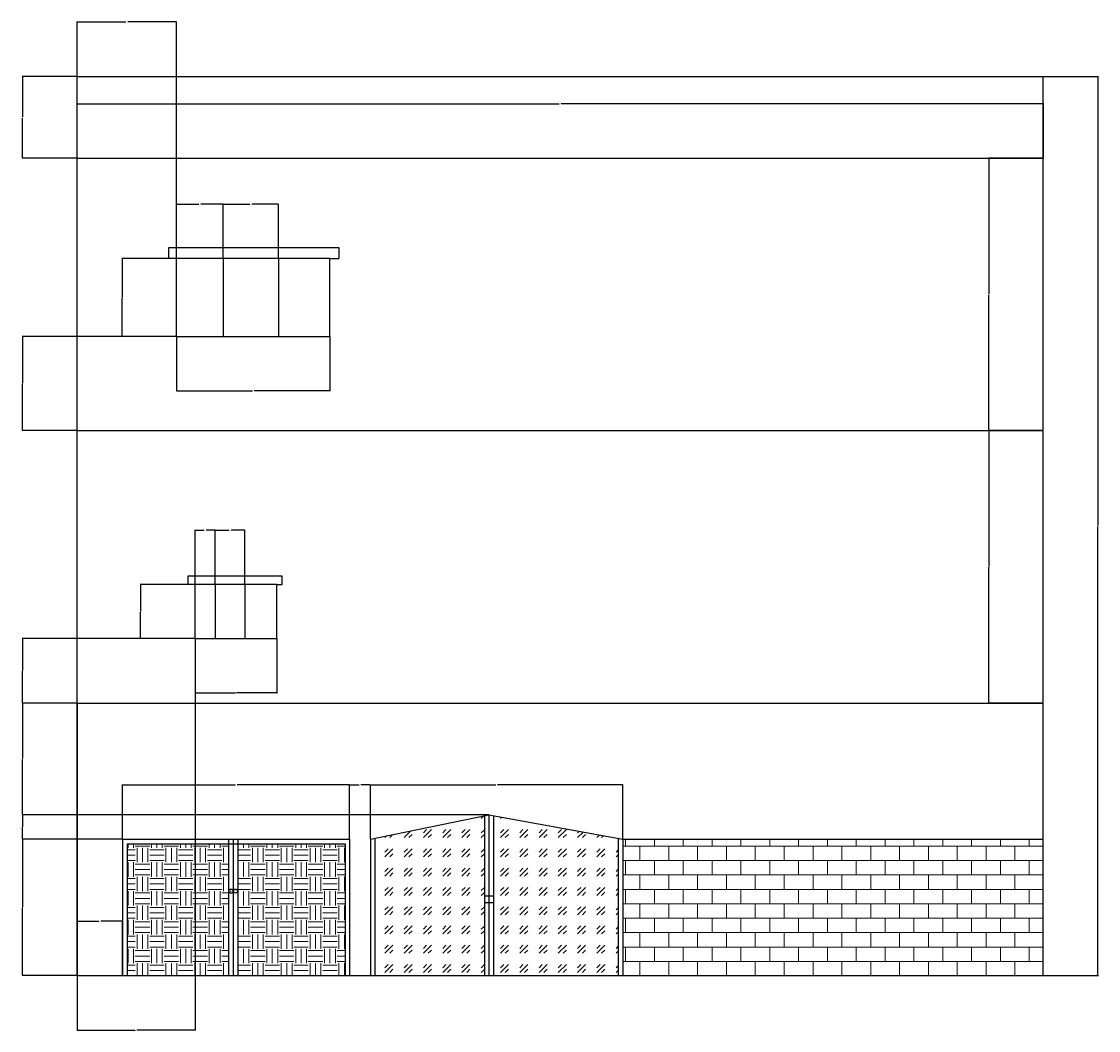
# Model space of a CAD drawing. Units: inches. Extents: x -45 to 1424, y 648 to 1662.
# Tile 8 of 8: x 924 to 1398, y 1218 to 1662. Entities that reach past the tile are written whole.
import ezdxf

# ---------------------------------------------------------------- set-up
doc = ezdxf.new("R2010")
doc.units = ezdxf.units.IN
for name, color, linetype, lineweight in [('A-ANNO-DIMS', 2, 'Continuous', 18), ('A-ELEV', 7, 'Continuous', 25), ('A-ELEV-PATT', 6, 'Continuous', 13), ('A-WALL-PATT', 6, 'Continuous', 13)]:
    doc.layers.add(name, color=color, linetype=linetype, lineweight=lineweight)
doc.styles.get("Standard").update_dxf_attribs({"font": 'arial.ttf'})
doc.dimstyles.get("Standard").update_dxf_attribs({"dimtxt": 0.18, "dimasz": 0.18, "dimexe": 0.18, "dimexo": 0.0625, "dimgap": 0.09, "dimtad": 0, "dimtih": 1, "dimtoh": 1, "dimdec": 4, "dimzin": 0, "dimdsep": 46, "dimtxsty": 'Standard', "dimcen": 0.09, "dimadec": 0, "dimazin": 0, "dimtfac": 1, "dimtdec": 4, "dimtofl": 0, "dimtmove": 0, "dimatfit": 3, "dimfxl": 1, "dimtolj": 1, "dimtzin": 0, "dimarcsym": 0})

# ---------------------------------------------------------------- blocks, each defined once
blk = doc.blocks.new('*D118')
at = {"layer": 'A-ANNO-DIMS', "color": 0, "lineweight": -2, "transparency": 16777216}
for p, q in [((948.45, 1602.23), (948.45, 1626.35)), ((948.63, 1626.17), (1160.84, 1626.17)), ((1373.85, 1626.17), (1161.63, 1626.17)), ((1374.03, 1602.23), (1374.03, 1626.35))]:
    blk.add_line(p, q, dxfattribs=at)
at = {"layer": 'A-ANNO-DIMS', "color": 0, "transparency": 16777216}
for points in [[(948.63, 1626.2), (948.63, 1626.14), (948.45, 1626.17)], [(1373.85, 1626.2), (1373.85, 1626.14), (1374.03, 1626.17)]]:
    blk.add_solid(points, dxfattribs=at)
at = {"layer": 'Defpoints', "color": 0, "transparency": 16777216}
for p in [(1374.03, 1626.17), (948.45, 1602.17), (1374.03, 1602.17)]:
    blk.add_point(p, dxfattribs=at)
at = {"layer": 'A-ANNO-DIMS', "color": 0, "transparency": 16777216, "insert": (1161.24, 1626.17), "char_height": 0.18, "attachment_point": 5}
blk.add_mtext('\\A1;425.6', dxfattribs=at)
blk = doc.blocks.new('*D119')
at = {"layer": 'A-ANNO-DIMS', "color": 0, "lineweight": -2, "transparency": 16777216}
for p, q in [((1374.09, 1638.17), (1398.21, 1638.17)), ((1398.03, 1637.99), (1398.03, 1440.35)), ((1398.03, 1242.35), (1398.03, 1439.98)), ((1374.09, 1242.17), (1398.21, 1242.17))]:
    blk.add_line(p, q, dxfattribs=at)
at = {"layer": 'A-ANNO-DIMS', "color": 0, "transparency": 16777216}
for points in [[(1398, 1637.99), (1398.06, 1637.99), (1398.03, 1638.17)], [(1398, 1242.35), (1398.06, 1242.35), (1398.03, 1242.17)]]:
    blk.add_solid(points, dxfattribs=at)
at = {"layer": 'Defpoints', "color": 0, "transparency": 16777216}
for p in [(1374.03, 1638.17), (1398.03, 1638.17), (1374.03, 1242.17)]:
    blk.add_point(p, dxfattribs=at)
at = {"layer": 'A-ANNO-DIMS', "color": 0, "transparency": 16777216, "insert": (1398.03, 1440.17), "char_height": 0.18, "attachment_point": 5}
blk.add_mtext('\\A1;396', dxfattribs=at)
blk = doc.blocks.new('*D120')
at = {"layer": 'A-ANNO-DIMS', "color": 0, "lineweight": -2, "transparency": 16777216}
for p, q in [((968.48, 1302.17), (924.27, 1302.17)), ((924.45, 1301.99), (924.45, 1272.35)), ((924.45, 1242.35), (924.45, 1271.98)), ((948.38, 1242.17), (924.27, 1242.17))]:
    blk.add_line(p, q, dxfattribs=at)
at = {"layer": 'A-ANNO-DIMS', "color": 0, "transparency": 16777216}
for points in [[(924.42, 1301.99), (924.48, 1301.99), (924.45, 1302.17)], [(924.42, 1242.35), (924.48, 1242.35), (924.45, 1242.17)]]:
    blk.add_solid(points, dxfattribs=at)
at = {"layer": 'Defpoints', "color": 0, "transparency": 16777216}
for p in [(924.45, 1302.17), (968.54, 1302.17), (948.45, 1242.17)]:
    blk.add_point(p, dxfattribs=at)
at = {"layer": 'A-ANNO-DIMS', "color": 0, "transparency": 16777216, "insert": (924.45, 1272.17), "char_height": 0.18, "attachment_point": 5}
blk.add_mtext('\\A1;60', dxfattribs=at)
blk = doc.blocks.new('*D121')
at = {"layer": 'A-ANNO-DIMS', "color": 0, "lineweight": -2, "transparency": 16777216}
for p, q in [((1129.76, 1312.93), (924.27, 1312.93)), ((924.45, 1312.75), (924.45, 1307.73)), ((924.45, 1302.35), (924.45, 1307.37)), ((968.48, 1302.17), (924.27, 1302.17))]:
    blk.add_line(p, q, dxfattribs=at)
at = {"layer": 'A-ANNO-DIMS', "color": 0, "transparency": 16777216}
for points in [[(924.42, 1312.75), (924.48, 1312.75), (924.45, 1312.93)], [(924.42, 1302.35), (924.48, 1302.35), (924.45, 1302.17)]]:
    blk.add_solid(points, dxfattribs=at)
at = {"layer": 'Defpoints', "color": 0, "transparency": 16777216}
for p in [(924.45, 1312.93), (1129.83, 1312.93), (968.54, 1302.17)]:
    blk.add_point(p, dxfattribs=at)
at = {"layer": 'A-ANNO-DIMS', "color": 0, "transparency": 16777216, "insert": (924.45, 1307.55), "char_height": 0.18, "attachment_point": 5}
blk.add_mtext('\\A1;10.769', dxfattribs=at)
blk = doc.blocks.new('*D122')
at = {"layer": 'A-ANNO-DIMS', "color": 0, "lineweight": -2, "transparency": 16777216}
for p, q in [((948.38, 1362.17), (924.27, 1362.17)), ((924.45, 1361.99), (924.45, 1337.73)), ((924.45, 1313.11), (924.45, 1337.37)), ((1129.76, 1312.93), (924.27, 1312.93))]:
    blk.add_line(p, q, dxfattribs=at)
at = {"layer": 'A-ANNO-DIMS', "color": 0, "transparency": 16777216}
for points in [[(924.42, 1361.99), (924.48, 1361.99), (924.45, 1362.17)], [(924.42, 1313.11), (924.48, 1313.11), (924.45, 1312.93)]]:
    blk.add_solid(points, dxfattribs=at)
at = {"layer": 'Defpoints', "color": 0, "transparency": 16777216}
for p in [(924.45, 1362.17), (948.45, 1362.17), (1129.83, 1312.93)]:
    blk.add_point(p, dxfattribs=at)
at = {"layer": 'A-ANNO-DIMS', "color": 0, "transparency": 16777216, "insert": (924.45, 1337.55), "char_height": 0.18, "attachment_point": 5}
blk.add_mtext('\\A1;49.23', dxfattribs=at)
blk = doc.blocks.new('*D123')
at = {"layer": 'A-ANNO-DIMS', "color": 0, "lineweight": -2, "transparency": 16777216}
for p, q in [((1373.96, 1482.17), (1349.85, 1482.17)), ((1350.03, 1481.99), (1350.03, 1422.35)), ((1350.03, 1362.35), (1350.03, 1421.98)), ((1373.96, 1362.17), (1349.85, 1362.17))]:
    blk.add_line(p, q, dxfattribs=at)
at = {"layer": 'A-ANNO-DIMS', "color": 0, "transparency": 16777216}
for points in [[(1350, 1481.99), (1350.06, 1481.99), (1350.03, 1482.17)], [(1350, 1362.35), (1350.06, 1362.35), (1350.03, 1362.17)]]:
    blk.add_solid(points, dxfattribs=at)
at = {"layer": 'Defpoints', "color": 0, "transparency": 16777216}
for p in [(1350.03, 1482.17), (1374.03, 1482.17), (1374.03, 1362.17)]:
    blk.add_point(p, dxfattribs=at)
at = {"layer": 'A-ANNO-DIMS', "color": 0, "transparency": 16777216, "insert": (1350.03, 1422.17), "char_height": 0.18, "attachment_point": 5}
blk.add_mtext('\\A1;120', dxfattribs=at)
blk = doc.blocks.new('*D124')
at = {"layer": 'A-ANNO-DIMS', "color": 0, "lineweight": -2, "transparency": 16777216}
for p, q in [((1373.96, 1602.17), (1349.85, 1602.17)), ((1350.03, 1601.99), (1350.03, 1542.35)), ((1350.03, 1482.35), (1350.03, 1541.98)), ((1373.96, 1482.17), (1349.85, 1482.17))]:
    blk.add_line(p, q, dxfattribs=at)
at = {"layer": 'A-ANNO-DIMS', "color": 0, "transparency": 16777216}
for points in [[(1350, 1601.99), (1350.06, 1601.99), (1350.03, 1602.17)], [(1350, 1482.35), (1350.06, 1482.35), (1350.03, 1482.17)]]:
    blk.add_solid(points, dxfattribs=at)
at = {"layer": 'Defpoints', "color": 0, "transparency": 16777216}
for p in [(1350.03, 1602.17), (1374.03, 1602.17), (1374.03, 1482.17)]:
    blk.add_point(p, dxfattribs=at)
at = {"layer": 'A-ANNO-DIMS', "color": 0, "transparency": 16777216, "insert": (1350.03, 1542.17), "char_height": 0.18, "attachment_point": 5}
blk.add_mtext('\\A1;120', dxfattribs=at)
blk = doc.blocks.new('*D125')
at = {"layer": 'A-ANNO-DIMS', "color": 0, "lineweight": -2, "transparency": 16777216}
for p, q in [((948.38, 1638.17), (924.27, 1638.17)), ((924.45, 1637.99), (924.45, 1620.35)), ((924.45, 1602.35), (924.45, 1619.98)), ((948.38, 1602.17), (924.27, 1602.17))]:
    blk.add_line(p, q, dxfattribs=at)
at = {"layer": 'A-ANNO-DIMS', "color": 0, "transparency": 16777216}
for points in [[(924.42, 1637.99), (924.48, 1637.99), (924.45, 1638.17)], [(924.42, 1602.35), (924.48, 1602.35), (924.45, 1602.17)]]:
    blk.add_solid(points, dxfattribs=at)
at = {"layer": 'Defpoints', "color": 0, "transparency": 16777216}
for p in [(924.45, 1638.17), (948.45, 1638.17), (948.45, 1602.17)]:
    blk.add_point(p, dxfattribs=at)
at = {"layer": 'A-ANNO-DIMS', "color": 0, "transparency": 16777216, "insert": (924.45, 1620.17), "char_height": 0.18, "attachment_point": 5}
blk.add_mtext('\\A1;36', dxfattribs=at)
blk = doc.blocks.new('*D126')
at = {"layer": 'A-ANNO-DIMS', "color": 0, "lineweight": -2, "transparency": 16777216}
for p, q in [((948.45, 1242.23), (948.45, 1266.35)), ((968.54, 1242.23), (968.54, 1266.35)), ((948.63, 1266.17), (958.03, 1266.17)), ((968.36, 1266.17), (958.96, 1266.17))]:
    blk.add_line(p, q, dxfattribs=at)
at = {"layer": 'A-ANNO-DIMS', "color": 0, "transparency": 16777216}
for points in [[(948.63, 1266.2), (948.63, 1266.14), (948.45, 1266.17)], [(968.36, 1266.2), (968.36, 1266.14), (968.54, 1266.17)]]:
    blk.add_solid(points, dxfattribs=at)
at = {"layer": 'Defpoints', "color": 0, "transparency": 16777216}
for p in [(968.54, 1266.17), (948.45, 1242.17), (968.54, 1242.17)]:
    blk.add_point(p, dxfattribs=at)
at = {"layer": 'A-ANNO-DIMS', "color": 0, "transparency": 16777216, "insert": (958.49, 1266.17), "char_height": 0.18, "attachment_point": 5}
blk.add_mtext('\\A1;20.095', dxfattribs=at)
blk = doc.blocks.new('*D127')
at = {"layer": 'A-ANNO-DIMS', "color": 0, "lineweight": -2, "transparency": 16777216}
for p, q in [((968.54, 1302.23), (968.54, 1326.35)), ((968.72, 1326.17), (1018.11, 1326.17)), ((1068.29, 1326.17), (1018.9, 1326.17)), ((1068.47, 1302.23), (1068.47, 1326.35))]:
    blk.add_line(p, q, dxfattribs=at)
at = {"layer": 'A-ANNO-DIMS', "color": 0, "transparency": 16777216}
for points in [[(968.72, 1326.2), (968.72, 1326.14), (968.54, 1326.17)], [(1068.29, 1326.2), (1068.29, 1326.14), (1068.47, 1326.17)]]:
    blk.add_solid(points, dxfattribs=at)
at = {"layer": 'Defpoints', "color": 0, "transparency": 16777216}
for p in [(1068.47, 1326.17), (968.54, 1302.17), (1068.47, 1302.17)]:
    blk.add_point(p, dxfattribs=at)
at = {"layer": 'A-ANNO-DIMS', "color": 0, "transparency": 16777216, "insert": (1018.51, 1326.17), "char_height": 0.18, "attachment_point": 5}
blk.add_mtext('\\A1;99.93', dxfattribs=at)
blk = doc.blocks.new('*D128')
at = {"layer": 'A-ANNO-DIMS', "color": 0, "lineweight": -2, "transparency": 16777216}
for p, q in [((1068.47, 1302.23), (1068.47, 1326.35)), ((1068.65, 1326.17), (1072.65, 1326.17)), ((1077.44, 1326.17), (1073.44, 1326.17)), ((1077.62, 1302.23), (1077.62, 1326.35))]:
    blk.add_line(p, q, dxfattribs=at)
at = {"layer": 'A-ANNO-DIMS', "color": 0, "transparency": 16777216}
for points in [[(1068.65, 1326.2), (1068.65, 1326.14), (1068.47, 1326.17)], [(1077.44, 1326.2), (1077.44, 1326.14), (1077.62, 1326.17)]]:
    blk.add_solid(points, dxfattribs=at)
at = {"layer": 'Defpoints', "color": 0, "transparency": 16777216}
for p in [(1077.62, 1326.17), (1068.47, 1302.17), (1077.62, 1302.17)]:
    blk.add_point(p, dxfattribs=at)
at = {"layer": 'A-ANNO-DIMS', "color": 0, "transparency": 16777216, "insert": (1073.05, 1326.17), "char_height": 0.18, "attachment_point": 5}
blk.add_mtext('\\A1;9.149', dxfattribs=at)
blk = doc.blocks.new('*D129')
at = {"layer": 'A-ANNO-DIMS', "color": 0, "lineweight": -2, "transparency": 16777216}
for p, q in [((1077.62, 1302.23), (1077.62, 1326.35)), ((1077.8, 1326.17), (1132.83, 1326.17)), ((1188.63, 1326.17), (1133.6, 1326.17)), ((1188.81, 1302.23), (1188.81, 1326.35))]:
    blk.add_line(p, q, dxfattribs=at)
at = {"layer": 'A-ANNO-DIMS', "color": 0, "transparency": 16777216}
for points in [[(1077.8, 1326.2), (1077.8, 1326.14), (1077.62, 1326.17)], [(1188.63, 1326.2), (1188.63, 1326.14), (1188.81, 1326.17)]]:
    blk.add_solid(points, dxfattribs=at)
at = {"layer": 'Defpoints', "color": 0, "transparency": 16777216}
for p in [(1188.81, 1326.17), (1077.62, 1302.17), (1188.81, 1302.17)]:
    blk.add_point(p, dxfattribs=at)
at = {"layer": 'A-ANNO-DIMS', "color": 0, "transparency": 16777216, "insert": (1133.22, 1326.17), "char_height": 0.18, "attachment_point": 5}
blk.add_mtext('\\A1;111.2', dxfattribs=at)
blk = doc.blocks.new('*D130')
at = {"layer": 'A-ANNO-DIMS', "color": 0, "lineweight": -2, "transparency": 16777216}
for p, q in [((1000.44, 1390.56), (1000.44, 1366.44)), ((1036.44, 1390.56), (1036.44, 1366.44)), ((1000.62, 1366.62), (1018.22, 1366.62)), ((1036.26, 1366.62), (1018.66, 1366.62))]:
    blk.add_line(p, q, dxfattribs=at)
at = {"layer": 'A-ANNO-DIMS', "color": 0, "transparency": 16777216}
for points in [[(1000.62, 1366.65), (1000.62, 1366.59), (1000.44, 1366.62)], [(1036.26, 1366.65), (1036.26, 1366.59), (1036.44, 1366.62)]]:
    blk.add_solid(points, dxfattribs=at)
at = {"layer": 'Defpoints', "color": 0, "transparency": 16777216}
for p in [(1000.44, 1390.62), (1036.44, 1390.62), (1000.44, 1366.62)]:
    blk.add_point(p, dxfattribs=at)
at = {"layer": 'A-ANNO-DIMS', "color": 0, "transparency": 16777216, "insert": (1018.44, 1366.62), "char_height": 0.18, "attachment_point": 5}
blk.add_mtext('\\A1;36', dxfattribs=at)
blk = doc.blocks.new('*D131')
at = {"layer": 'A-ANNO-DIMS', "color": 0, "lineweight": -2, "transparency": 16777216}
for p, q in [((1000.44, 1390.56), (1000.44, 1217.99)), ((948.45, 1362.1), (948.45, 1217.99)), ((948.63, 1218.17), (974.05, 1218.17)), ((1000.26, 1218.17), (974.84, 1218.17))]:
    blk.add_line(p, q, dxfattribs=at)
at = {"layer": 'A-ANNO-DIMS', "color": 0, "transparency": 16777216}
for points in [[(948.63, 1218.2), (948.63, 1218.14), (948.45, 1218.17)], [(1000.26, 1218.2), (1000.26, 1218.14), (1000.44, 1218.17)]]:
    blk.add_solid(points, dxfattribs=at)
at = {"layer": 'Defpoints', "color": 0, "transparency": 16777216}
for p in [(1000.44, 1390.62), (948.45, 1362.17), (1000.44, 1218.17)]:
    blk.add_point(p, dxfattribs=at)
at = {"layer": 'A-ANNO-DIMS', "color": 0, "transparency": 16777216, "insert": (974.44, 1218.17), "char_height": 0.18, "attachment_point": 5}
blk.add_mtext('\\A1;51.99', dxfattribs=at)
blk = doc.blocks.new('*D132')
at = {"layer": 'A-ANNO-DIMS', "color": 0, "lineweight": -2, "transparency": 16777216}
for p, q in [((1000.38, 1390.62), (924.27, 1390.62)), ((924.45, 1390.44), (924.45, 1376.57)), ((924.45, 1362.35), (924.45, 1376.21)), ((948.38, 1362.17), (924.27, 1362.17))]:
    blk.add_line(p, q, dxfattribs=at)
at = {"layer": 'A-ANNO-DIMS', "color": 0, "transparency": 16777216}
for points in [[(924.42, 1390.44), (924.48, 1390.44), (924.45, 1390.62)], [(924.42, 1362.35), (924.48, 1362.35), (924.45, 1362.17)]]:
    blk.add_solid(points, dxfattribs=at)
at = {"layer": 'Defpoints', "color": 0, "transparency": 16777216}
for p in [(924.45, 1390.62), (1000.44, 1390.62), (948.45, 1362.17)]:
    blk.add_point(p, dxfattribs=at)
at = {"layer": 'A-ANNO-DIMS', "color": 0, "transparency": 16777216, "insert": (924.45, 1376.39), "char_height": 0.18, "attachment_point": 5}
blk.add_mtext('\\A1;28.455', dxfattribs=at)
blk = doc.blocks.new('*D133')
at = {"layer": 'A-ANNO-DIMS', "color": 0, "lineweight": -2, "transparency": 16777216}
for p, q in [((1000.38, 1414.33), (976.26, 1414.33)), ((976.44, 1414.15), (976.44, 1402.66)), ((976.44, 1390.8), (976.44, 1402.29)), ((1000.38, 1390.62), (976.26, 1390.62))]:
    blk.add_line(p, q, dxfattribs=at)
at = {"layer": 'A-ANNO-DIMS', "color": 0, "transparency": 16777216}
for points in [[(976.41, 1414.15), (976.47, 1414.15), (976.44, 1414.33)], [(976.41, 1390.8), (976.47, 1390.8), (976.44, 1390.62)]]:
    blk.add_solid(points, dxfattribs=at)
at = {"layer": 'Defpoints', "color": 0, "transparency": 16777216}
for p in [(976.44, 1414.33), (1000.44, 1414.33), (1000.44, 1390.62)]:
    blk.add_point(p, dxfattribs=at)
at = {"layer": 'A-ANNO-DIMS', "color": 0, "transparency": 16777216, "insert": (976.44, 1402.47), "char_height": 0.18, "attachment_point": 5}
blk.add_mtext('\\A1;23.71', dxfattribs=at)
blk = doc.blocks.new('*D134')
at = {"layer": 'A-ANNO-DIMS', "color": 0, "lineweight": -2, "transparency": 16777216}
for p, q in [((992.29, 1523.6), (992.29, 1499.49)), ((1059.83, 1523.6), (1059.83, 1499.49)), ((992.47, 1499.67), (1025.67, 1499.67)), ((1059.65, 1499.67), (1026.45, 1499.67))]:
    blk.add_line(p, q, dxfattribs=at)
at = {"layer": 'A-ANNO-DIMS', "color": 0, "transparency": 16777216}
for points in [[(992.47, 1499.7), (992.47, 1499.64), (992.29, 1499.67)], [(1059.65, 1499.7), (1059.65, 1499.64), (1059.83, 1499.67)]]:
    blk.add_solid(points, dxfattribs=at)
at = {"layer": 'Defpoints', "color": 0, "transparency": 16777216}
for p in [(992.29, 1523.67), (1059.83, 1523.67), (992.29, 1499.67)]:
    blk.add_point(p, dxfattribs=at)
at = {"layer": 'A-ANNO-DIMS', "color": 0, "transparency": 16777216, "insert": (1026.06, 1499.67), "char_height": 0.18, "attachment_point": 5}
blk.add_mtext('\\A1;67.54', dxfattribs=at)
blk = doc.blocks.new('*D135')
at = {"layer": 'A-ANNO-DIMS', "color": 0, "lineweight": -2, "transparency": 16777216}
for p, q in [((948.45, 1482.23), (948.45, 1662.35)), ((948.63, 1662.17), (969.97, 1662.17)), ((992.11, 1662.17), (970.77, 1662.17)), ((992.29, 1523.73), (992.29, 1662.35))]:
    blk.add_line(p, q, dxfattribs=at)
at = {"layer": 'A-ANNO-DIMS', "color": 0, "transparency": 16777216}
for points in [[(948.63, 1662.2), (948.63, 1662.14), (948.45, 1662.17)], [(992.11, 1662.2), (992.11, 1662.14), (992.29, 1662.17)]]:
    blk.add_solid(points, dxfattribs=at)
at = {"layer": 'Defpoints', "color": 0, "transparency": 16777216}
for p in [(992.29, 1662.17), (992.29, 1523.67), (948.45, 1482.17)]:
    blk.add_point(p, dxfattribs=at)
at = {"layer": 'A-ANNO-DIMS', "color": 0, "transparency": 16777216, "insert": (970.37, 1662.17), "char_height": 0.18, "attachment_point": 5}
blk.add_mtext('\\A1;43.85', dxfattribs=at)
blk = doc.blocks.new('*D136')
at = {"layer": 'A-ANNO-DIMS', "color": 0, "lineweight": -2, "transparency": 16777216}
for p, q in [((992.23, 1523.67), (924.27, 1523.67)), ((924.45, 1523.49), (924.45, 1503.1)), ((924.45, 1482.35), (924.45, 1502.73)), ((948.38, 1482.17), (924.27, 1482.17))]:
    blk.add_line(p, q, dxfattribs=at)
at = {"layer": 'A-ANNO-DIMS', "color": 0, "transparency": 16777216}
for points in [[(924.42, 1523.49), (924.48, 1523.49), (924.45, 1523.67)], [(924.42, 1482.35), (924.48, 1482.35), (924.45, 1482.17)]]:
    blk.add_solid(points, dxfattribs=at)
at = {"layer": 'Defpoints', "color": 0, "transparency": 16777216}
for p in [(924.45, 1523.67), (992.29, 1523.67), (948.45, 1482.17)]:
    blk.add_point(p, dxfattribs=at)
at = {"layer": 'A-ANNO-DIMS', "color": 0, "transparency": 16777216, "insert": (924.45, 1502.92), "char_height": 0.18, "attachment_point": 5}
blk.add_mtext('\\A1;41.5', dxfattribs=at)
blk = doc.blocks.new('*D137')
at = {"layer": 'A-ANNO-DIMS', "color": 0, "lineweight": -2, "transparency": 16777216}
for p, q in [((992.23, 1557.91), (968.11, 1557.91)), ((968.29, 1557.73), (968.29, 1540.97)), ((968.29, 1523.85), (968.29, 1540.61)), ((992.23, 1523.67), (968.11, 1523.67))]:
    blk.add_line(p, q, dxfattribs=at)
at = {"layer": 'A-ANNO-DIMS', "color": 0, "transparency": 16777216}
for points in [[(968.26, 1557.73), (968.32, 1557.73), (968.29, 1557.91)], [(968.26, 1523.85), (968.32, 1523.85), (968.29, 1523.67)]]:
    blk.add_solid(points, dxfattribs=at)
at = {"layer": 'Defpoints', "color": 0, "transparency": 16777216}
for p in [(968.29, 1557.91), (992.29, 1557.91), (992.29, 1523.67)]:
    blk.add_point(p, dxfattribs=at)
at = {"layer": 'A-ANNO-DIMS', "color": 0, "transparency": 16777216, "insert": (968.29, 1540.79), "char_height": 0.18, "attachment_point": 5}
blk.add_mtext('\\A1;34.245', dxfattribs=at)
blk = doc.blocks.new('*D138')
at = {"layer": 'A-ANNO-DIMS', "color": 0, "lineweight": -2, "transparency": 16777216}
for p, q in [((992.29, 1557.97), (992.29, 1582.09)), ((992.47, 1581.91), (1002.1, 1581.91)), ((1012.66, 1581.91), (1003.03, 1581.91)), ((1012.84, 1557.97), (1012.84, 1582.09))]:
    blk.add_line(p, q, dxfattribs=at)
at = {"layer": 'A-ANNO-DIMS', "color": 0, "transparency": 16777216}
for points in [[(992.47, 1581.94), (992.47, 1581.88), (992.29, 1581.91)], [(1012.66, 1581.94), (1012.66, 1581.88), (1012.84, 1581.91)]]:
    blk.add_solid(points, dxfattribs=at)
at = {"layer": 'Defpoints', "color": 0, "transparency": 16777216}
for p in [(1012.84, 1581.91), (992.29, 1557.91), (1012.84, 1557.91)]:
    blk.add_point(p, dxfattribs=at)
at = {"layer": 'A-ANNO-DIMS', "color": 0, "transparency": 16777216, "insert": (1002.56, 1581.91), "char_height": 0.18, "attachment_point": 5}
blk.add_mtext('\\A1;20.546', dxfattribs=at)
blk = doc.blocks.new('*D139')
at = {"layer": 'A-ANNO-DIMS', "color": 0, "lineweight": -2, "transparency": 16777216}
for p, q in [((1012.84, 1557.97), (1012.84, 1582.09)), ((1013.02, 1581.91), (1024.58, 1581.91)), ((1036.94, 1581.91), (1025.37, 1581.91)), ((1037.12, 1557.97), (1037.12, 1582.09))]:
    blk.add_line(p, q, dxfattribs=at)
at = {"layer": 'A-ANNO-DIMS', "color": 0, "transparency": 16777216}
for points in [[(1013.02, 1581.94), (1013.02, 1581.88), (1012.84, 1581.91)], [(1036.94, 1581.94), (1036.94, 1581.88), (1037.12, 1581.91)]]:
    blk.add_solid(points, dxfattribs=at)
at = {"layer": 'Defpoints', "color": 0, "transparency": 16777216}
for p in [(1037.12, 1581.91), (1012.84, 1557.91), (1037.12, 1557.91)]:
    blk.add_point(p, dxfattribs=at)
at = {"layer": 'A-ANNO-DIMS', "color": 0, "transparency": 16777216, "insert": (1024.98, 1581.91), "char_height": 0.18, "attachment_point": 5}
blk.add_mtext('\\A1;24.28', dxfattribs=at)
blk = doc.blocks.new('*D140')
at = {"layer": 'A-ANNO-DIMS', "color": 0, "lineweight": -2, "transparency": 16777216}
for p, q in [((1000.44, 1414.39), (1000.44, 1438.51)), ((1000.62, 1438.33), (1004.47, 1438.33)), ((1009.12, 1438.33), (1005.26, 1438.33)), ((1009.3, 1414.39), (1009.3, 1438.51))]:
    blk.add_line(p, q, dxfattribs=at)
at = {"layer": 'A-ANNO-DIMS', "color": 0, "transparency": 16777216}
for points in [[(1000.62, 1438.36), (1000.62, 1438.3), (1000.44, 1438.33)], [(1009.12, 1438.36), (1009.12, 1438.3), (1009.3, 1438.33)]]:
    blk.add_solid(points, dxfattribs=at)
at = {"layer": 'Defpoints', "color": 0, "transparency": 16777216}
for p in [(1009.3, 1438.33), (1000.44, 1414.33), (1009.3, 1414.33)]:
    blk.add_point(p, dxfattribs=at)
at = {"layer": 'A-ANNO-DIMS', "color": 0, "transparency": 16777216, "insert": (1004.87, 1438.33), "char_height": 0.18, "attachment_point": 5}
blk.add_mtext('\\A1;8.858', dxfattribs=at)
blk = doc.blocks.new('*D141')
at = {"layer": 'A-ANNO-DIMS', "color": 0, "lineweight": -2, "transparency": 16777216}
for p, q in [((1009.3, 1414.39), (1009.3, 1438.51)), ((1009.48, 1438.33), (1015.4, 1438.33)), ((1022.2, 1438.33), (1016.28, 1438.33)), ((1022.38, 1414.39), (1022.38, 1438.51))]:
    blk.add_line(p, q, dxfattribs=at)
at = {"layer": 'A-ANNO-DIMS', "color": 0, "transparency": 16777216}
for points in [[(1009.48, 1438.36), (1009.48, 1438.3), (1009.3, 1438.33)], [(1022.2, 1438.36), (1022.2, 1438.3), (1022.38, 1438.33)]]:
    blk.add_solid(points, dxfattribs=at)
at = {"layer": 'Defpoints', "color": 0, "transparency": 16777216}
for p in [(1022.38, 1438.33), (1009.3, 1414.33), (1022.38, 1414.33)]:
    blk.add_point(p, dxfattribs=at)
at = {"layer": 'A-ANNO-DIMS', "color": 0, "transparency": 16777216, "insert": (1015.84, 1438.33), "char_height": 0.18, "attachment_point": 5}
blk.add_mtext('\\A1;13.081', dxfattribs=at)
blk = doc.blocks.new('*D142')
at = {"layer": 'A-ANNO-DIMS', "color": 0, "lineweight": -2, "transparency": 16777216}
for p, q in [((1016.13, 1279.33), (1016.31, 1279.33)), ((1016.22, 1279.24), (1016.22, 1279.42)), ((1017.64, 1279.45), (1017.29, 1279.42))]:
    blk.add_line(p, q, dxfattribs=at)
at = {"layer": 'A-ANNO-DIMS', "color": 0, "transparency": 16777216}
blk.add_solid([(1017.29, 1279.45), (1017.29, 1279.39), (1017.11, 1279.41)], dxfattribs=at)
at = {"layer": 'Defpoints', "color": 0, "transparency": 16777216}
for p in [(1015.34, 1279.26), (1017.11, 1279.41)]:
    blk.add_point(p, dxfattribs=at)
at = {"layer": 'A-ANNO-DIMS', "color": 0, "transparency": 16777216, "insert": (1018.32, 1279.45), "char_height": 0.18, "attachment_point": 5}
blk.add_mtext('\\A1;2X ∅1.776', dxfattribs=at)

msp = doc.modelspace()

# ---------------------------------------------------------------- hatches: boundary and pattern name
at = {"layer": 'A-ELEV-PATT'}
h = msp.add_hatch(dxfattribs=at)
h.set_pattern_fill('GOST_GLASS', color=256)
h.set_pattern_definition([(45, (-2708.9, 1540.484), (8.485281, 0), [5, -7]), (45, (-2706.7786, 1540.484), (8.485281, 0), [2, -10]), (45, (-2708.9, 1542.6053), (8.485281, 0), [2, -10])])
h.paths.add_polyline_path([(1131.8269, 1242.165), (1186.8124, 1242.165), (1186.8124, 1302.5301), (1131.8269, 1312.5684)])
h.paths.add_polyline_path([(1127.8269, 1312.521), (1079.6208, 1302.5776), (1079.6208, 1242.165), (1127.8269, 1242.165)])
h = msp.add_hatch(dxfattribs=at)
h.set_pattern_fill('EARTH', color=256)
h.set_pattern_definition([(0, (-2708.9, 1540.484), (6.35, 6.35), [6.35, -6.35]), (0, (-2708.9, 1542.865), (6.35, 6.35), [6.35, -6.35]), (0, (-2708.9, 1545.2465), (6.35, 6.35), [6.35, -6.35]), (90, (-2708.106, 1546.04), (-6.35, 6.35), [6.35, -6.35]), (90, (-2705.725, 1546.04), (-6.35, 6.35), [6.35, -6.35]), (90, (-2703.3437, 1546.04), (-6.35, 6.35), [6.35, -6.35])])
h.paths.add_polyline_path([(1015.209, 1300.165), (970.5404, 1300.165), (970.5404, 1242.165), (1015.209, 1242.165)])
h.paths.add_polyline_path([(1019.209, 1242.165), (1066.4721, 1242.165), (1066.4721, 1300.165), (1019.209, 1300.165)])
at = {"layer": 'A-WALL-PATT'}
h = msp.add_hatch(dxfattribs=at)
h.set_pattern_fill('BRICK', color=256)
h.set_pattern_definition([(0, (-2708.9, 1540.484), (0, 6.35), []), (90, (-2708.9, 1540.484), (-12.7, 8e-16), [6.35, -6.35]), (90, (-2702.55, 1540.484), (-12.7, 8e-16), [-6.35, 6.35])])
h.paths.add_polyline_path([(1188.8124, 1302.165), (1188.8124, 1242.165), (1373.8453, 1242.165), (1373.8453, 1302.165)])

# ---------------------------------------------------------------- linework, layer by layer
at = {"layer": 'A-ELEV'}
for p, q in [((948.4453, 1242.165), (948.4453, 1638.165)), ((948.4453, 1638.165), (1374.0272, 1638.165)), ((1373.8453, 1242.165), (1373.8453, 1638.165)), ((948.4453, 1602.165), (1374.0272, 1602.165)), ((988.8705, 1557.9104), (988.8705, 1562.8441)), ((988.8705, 1562.8441), (1063.7076, 1562.8441)), ((1063.7076, 1562.8441), (1063.7076, 1557.9104)), ((992.2912, 1557.9104), (988.8705, 1557.9104)), ((1059.8291, 1557.9104), (992.2912, 1557.9104)), ((992.2912, 1523.6657), (992.2912, 1557.9104)), ((1012.8375, 1557.9104), (1012.8375, 1523.6657)), ((1037.1172, 1557.9104), (1037.1172, 1523.6657)), ((1059.8291, 1523.6657), (1059.8291, 1557.9104)), ((1059.8291, 1557.9104), (1063.7076, 1557.9104)), ((992.2912, 1523.6657), (1059.8291, 1523.6657)), ((948.4453, 1482.165), (1374.0272, 1482.165)), ((1038.8208, 1418.0224), (997.2967, 1418.0224)), ((997.2967, 1418.0224), (997.2967, 1414.3289)), ((1038.8208, 1414.3289), (1038.8208, 1418.0224)), ((1000.4401, 1414.3289), (997.2967, 1414.3289)), ((1036.4401, 1414.3289), (1000.4401, 1414.3289)), ((1000.4401, 1390.6196), (1000.4401, 1414.3289)), ((1009.2979, 1414.3289), (1009.2979, 1390.6196)), ((1022.3792, 1414.3289), (1022.3792, 1390.6196)), ((1036.4401, 1390.6196), (1036.4401, 1414.3289)), ((1036.4401, 1414.3289), (1038.8208, 1414.3289)), ((1000.4401, 1390.6196), (1036.4401, 1390.6196)), ((948.4453, 1362.165), (1374.0272, 1362.165)), ((1077.6208, 1302.165), (1129.8269, 1312.9335)), ((1127.8269, 1312.5952), (1127.8269, 1242.165)), ((1129.8269, 1312.9335), (1129.8269, 1242.165)), ((1129.8269, 1312.9335), (1188.8124, 1302.165)), ((1131.8269, 1312.5804), (1131.8269, 1242.165)), ((968.5404, 1302.165), (1068.4721, 1302.165)), ((968.5404, 1302.165), (968.5404, 1242.165)), ((970.5404, 1300.165), (970.5404, 1242.165)), ((970.5404, 1300.165), (1066.4721, 1300.165)), ((1015.209, 1302.165), (1015.209, 1242.165)), ((1017.209, 1302.165), (1017.209, 1242.165)), ((1019.209, 1302.165), (1019.209, 1242.165)), ((1019.209, 1302.165), (1019.209, 1242.165)), ((1019.209, 1302.165), (1019.209, 1242.165)), ((1066.4721, 1300.165), (1066.4721, 1242.165)), ((1068.4721, 1302.165), (1068.4721, 1242.165)), ((1077.6208, 1302.165), (1077.6208, 1242.165)), ((1079.6208, 1302.5776), (1079.6208, 1242.165)), ((1186.8124, 1302.5301), (1186.8124, 1242.165)), ((1188.8124, 1302.165), (1188.8124, 1242.165)), ((1188.8124, 1302.165), (1374.0272, 1302.165)), ((1127.8269, 1277.3227), (1131.8269, 1277.3227)), ((1127.8269, 1274.3227), (1131.8269, 1274.3227)), ((948.4453, 1242.165), (1374.0272, 1242.165))]:
    msp.add_line(p, q, dxfattribs=at)
for centre in [(1016.2243, 1279.3346), (1018.2211, 1279.3933)]:
    msp.add_circle(centre, 0.888, dxfattribs=at)

# ---------------------------------------------------------------- dimensions: what is measured, and where the dimension line sits
at = {"layer": 'A-ANNO-DIMS'}
for base, p1, p2, override, picture, middle in [((992.2912, 1662.165), (948.4453, 1482.165), (992.2912, 1523.6657), {"dimdec": 2, "dimlfac": 1, "dimrnd": 0, "dimzin": 0, "dimdsep": 46, "dimlunit": 2}, '*D135', (970.3683, 1662.165)), ((1374.0272, 1626.165), (948.4453, 1602.165), (1374.0272, 1602.165), {"dimdec": 1, "dimlfac": 1, "dimrnd": 0, "dimzin": 0, "dimdsep": 46, "dimlunit": 2}, '*D118', (1161.2362, 1626.165)), ((1012.8375, 1581.9104), (992.2912, 1557.9104), (1012.8375, 1557.9104), {"dimdec": 3, "dimlfac": 1, "dimrnd": 0, "dimzin": 0, "dimdsep": 46, "dimlunit": 2}, '*D138', (1002.5644, 1581.9104)), ((1037.1172, 1581.9104), (1012.8375, 1557.9104), (1037.1172, 1557.9104), {"dimdec": 2, "dimlfac": 1, "dimrnd": 0, "dimzin": 0, "dimdsep": 46, "dimlunit": 2}, '*D139', (1024.9774, 1581.9104)), ((1009.2979, 1438.3289), (1000.4401, 1414.3289), (1009.2979, 1414.3289), {"dimdec": 3, "dimlfac": 1, "dimrnd": 0, "dimzin": 0, "dimdsep": 46, "dimlunit": 2}, '*D140', (1004.869, 1438.3289)), ((1022.3792, 1438.3289), (1009.2979, 1414.3289), (1022.3792, 1414.3289), {"dimdec": 3, "dimlfac": 1, "dimrnd": 0, "dimzin": 0, "dimdsep": 46, "dimlunit": 2}, '*D141', (1015.8385, 1438.3289)), ((1000.4401, 1218.165), (948.4453, 1362.165), (1000.4401, 1390.6196), {"dimdec": 2, "dimlfac": 1, "dimrnd": 0, "dimzin": 0, "dimdsep": 46, "dimlunit": 2}, '*D131', (974.4427, 1218.165)), ((1068.4721, 1326.165), (968.5404, 1302.165), (1068.4721, 1302.165), {"dimdec": 2, "dimlfac": 1, "dimrnd": 0, "dimzin": 0, "dimdsep": 46, "dimlunit": 2}, '*D127', (1018.5062, 1326.165)), ((1077.6208, 1326.165), (1068.4721, 1302.165), (1077.6208, 1302.165), {"dimdec": 3, "dimlfac": 1, "dimrnd": 0, "dimzin": 0, "dimdsep": 46, "dimlunit": 2}, '*D128', (1073.0464, 1326.165)), ((1188.8124, 1326.165), (1077.6208, 1302.165), (1188.8124, 1302.165), {"dimdec": 1, "dimlfac": 1, "dimrnd": 0, "dimzin": 0, "dimdsep": 46, "dimlunit": 2}, '*D129', (1133.2166, 1326.165)), ((968.5404, 1266.165), (948.4453, 1242.165), (968.5404, 1242.165), {"dimdec": 3, "dimlfac": 1, "dimrnd": 0, "dimzin": 0, "dimdsep": 46, "dimlunit": 2}, '*D126', (958.4928, 1266.165))]:
    dim = msp.add_linear_dim(base=base, p1=p1, p2=p2, dimstyle='Standard', override=override, dxfattribs=at)
    dim.commit()
    dim.dimension.update_dxf_attribs({"geometry": picture, "text_midpoint": middle})
for base, p1, p2, angle, override, picture, middle in [((924.4453, 1638.165), (948.4453, 1602.165), (948.4453, 1638.165), 90, {"dimdec": 0, "dimlfac": 1, "dimrnd": 0, "dimzin": 0, "dimdsep": 46, "dimlunit": 2}, '*D125', (924.4453, 1620.165)), ((1398.0272, 1638.165), (1374.0272, 1242.165), (1374.0272, 1638.165), 90, {"dimdec": 0, "dimlfac": 1, "dimrnd": 0, "dimzin": 0, "dimdsep": 46, "dimlunit": 2}, '*D119', (1398.0272, 1440.165)), ((1350.0272, 1602.165), (1374.0272, 1482.165), (1374.0272, 1602.165), 90, {"dimdec": 0, "dimlfac": 1, "dimrnd": 0, "dimzin": 0, "dimdsep": 46, "dimlunit": 2}, '*D124', (1350.0272, 1542.165)), ((968.2912, 1557.9104), (992.2912, 1523.6657), (992.2912, 1557.9104), 90, {"dimdec": 3, "dimlfac": 1, "dimrnd": 0, "dimzin": 0, "dimdsep": 46, "dimlunit": 2}, '*D137', (968.2912, 1540.788)), ((924.4453, 1523.6657), (948.4453, 1482.165), (992.2912, 1523.6657), 90, {"dimdec": 1, "dimlfac": 1, "dimrnd": 0, "dimzin": 0, "dimdsep": 46, "dimlunit": 2}, '*D136', (924.4453, 1502.9153)), ((992.2912, 1499.6657), (1059.8291, 1523.6657), (992.2912, 1523.6657), 180, {"dimdec": 2, "dimlfac": 1, "dimrnd": 0, "dimzin": 0, "dimdsep": 46, "dimlunit": 2}, '*D134', (1026.0602, 1499.6657)), ((1350.0272, 1482.165), (1374.0272, 1362.165), (1374.0272, 1482.165), 90, {"dimdec": 0, "dimlfac": 1, "dimrnd": 0, "dimzin": 0, "dimdsep": 46, "dimlunit": 2}, '*D123', (1350.0272, 1422.165)), ((976.4401, 1414.3289), (1000.4401, 1390.6196), (1000.4401, 1414.3289), 90, {"dimdec": 2, "dimlfac": 1, "dimrnd": 0, "dimzin": 0, "dimdsep": 46, "dimlunit": 2}, '*D133', (976.4401, 1402.4742)), ((924.4453, 1390.6196), (948.4453, 1362.165), (1000.4401, 1390.6196), 90, {"dimdec": 3, "dimlfac": 1, "dimrnd": 0, "dimzin": 0, "dimdsep": 46, "dimlunit": 2}, '*D132', (924.4453, 1376.3923)), ((1000.4401, 1366.6196), (1036.4401, 1390.6196), (1000.4401, 1390.6196), 180, {"dimdec": 0, "dimlfac": 1, "dimrnd": 0, "dimzin": 0, "dimdsep": 46, "dimlunit": 2}, '*D130', (1018.4401, 1366.6196)), ((924.4453, 1362.165), (1129.8269, 1312.9335), (948.4453, 1362.165), 90, {"dimdec": 2, "dimlfac": 1, "dimrnd": 0, "dimzin": 0, "dimdsep": 46, "dimlunit": 2}, '*D122', (924.4453, 1337.5493)), ((924.44526, 1312.93355), (968.54036, 1302.16502), (1129.82688, 1312.93355), 90, {"dimdec": 3, "dimlfac": 1, "dimrnd": 0, "dimzin": 0, "dimdsep": 46, "dimlunit": 2}, '*D121', (924.44526, 1307.54929)), ((924.4453, 1302.165), (948.4453, 1242.165), (968.5404, 1302.165), 90, {"dimdec": 0, "dimlfac": 1, "dimrnd": 0, "dimzin": 0, "dimdsep": 46, "dimlunit": 2}, '*D120', (924.4453, 1272.165))]:
    dim = msp.add_linear_dim(base=base, p1=p1, p2=p2, angle=angle, dimstyle='Standard', override=override, dxfattribs=at)
    dim.commit()
    dim.dimension.update_dxf_attribs({"geometry": picture, "text_midpoint": middle})
dim = msp.add_diameter_dim_2p(p1=(1015.3395, 1279.26), p2=(1017.1092, 1279.4092), text='2X <>', dimstyle='Standard', override={"dimdec": 3, "dimlfac": 1, "dimrnd": 0, "dimzin": 0, "dimdsep": 46, "dimlunit": 2}, dxfattribs=at)
dim.commit()
dim.dimension.update_dxf_attribs({"geometry": '*D142', "text_midpoint": (1017.6401, 1279.454), "dimtype": 163})

doc.saveas('drawing.dxf')
